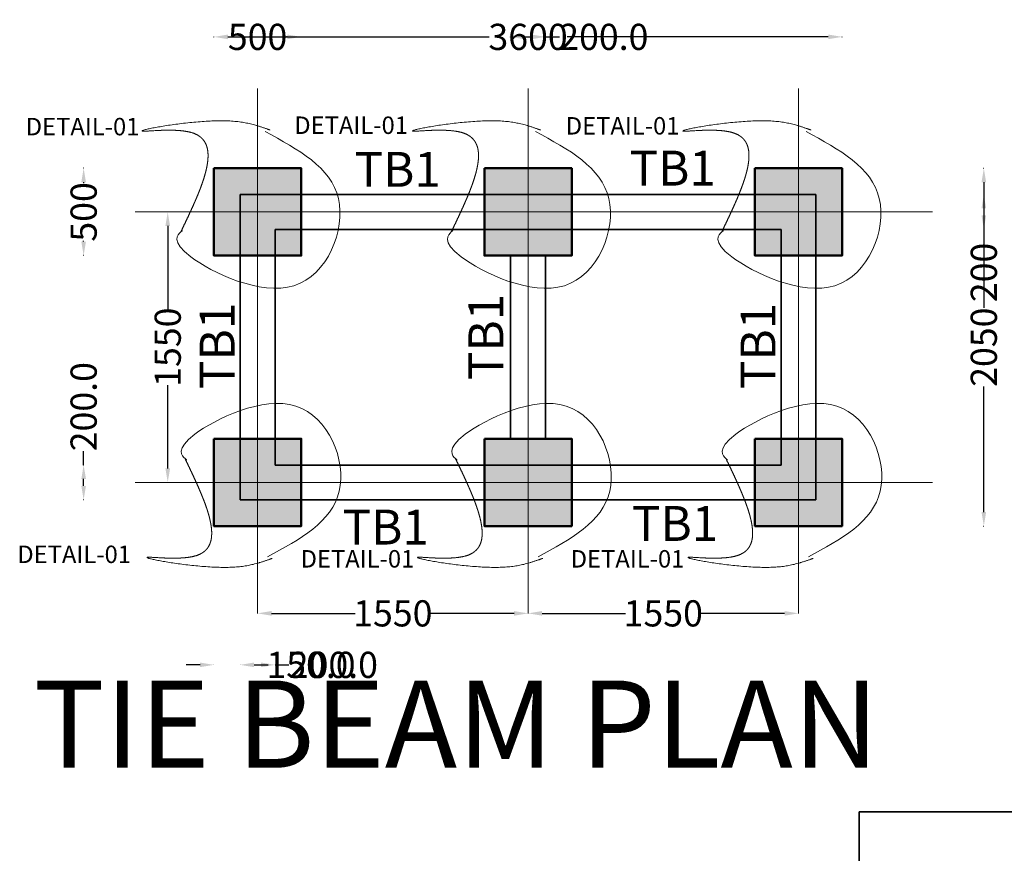
# Model space of a CAD drawing. Units: millimetres. Extents: x -19888 to 14444, y 67066 to 90098.
# Tile 5 of 7: x -13450 to -7807, y 82214 to 86990. Entities that reach past the tile are written whole.
import ezdxf

# ---------------------------------------------------------------- set-up
doc = ezdxf.new("R2010")
doc.units = ezdxf.units.MM
doc.header["$LTSCALE"] = 50
doc.header["$MEASUREMENT"] = 0
doc.linetypes.add('CENTER', pattern=[50.8, 31.75, -6.35, 6.35, -6.35])
for name, color, linetype, lineweight in [('S-ANNO-DIMS', 2, 'Continuous', 18), ('S-ANNO-SYMB', 3, 'Continuous', 18), ('S-ANNO-TEXT', 7, 'Continuous', 25), ('S-ANNO-TTLB', 7, 'Continuous', 35), ('S-BEAM', 3, 'Continuous', 35), ('S-COLS', 4, 'Continuous', 50), ('S-GRID', 8, 'CENTER', 18), ('S-PATT', 8, 'Continuous', 13)]:
    doc.layers.add(name, color=color, linetype=linetype, lineweight=lineweight)
doc.styles.get("Standard").update_dxf_attribs({"font": 'arial.ttf'})
doc.dimstyles.get("Standard").update_dxf_attribs({"dimtxt": 150, "dimasz": 80, "dimexe": 0.18, "dimexo": 0.0625, "dimgap": 0.09, "dimtad": 0, "dimdec": 0, "dimzin": 0, "dimdsep": 46, "dimtxsty": 'Standard', "dimcen": 0.09, "dimadec": 0, "dimazin": 0, "dimtfac": 1, "dimtdec": 0, "dimtofl": 0, "dimtmove": 0, "dimatfit": 3, "dimfxl": 1, "dimfxlon": 1, "dimtolj": 1, "dimtzin": 0, "dimarcsym": 0})

# ---------------------------------------------------------------- blocks, each defined once
blk = doc.blocks.new('*D16')
at = {"layer": 'Defpoints', "color": 0, "ltscale": 50, "transparency": 16777216}
for p in [(-12086.8, 83589.1), (-10536.8, 83589.1), (-10536.8, 83589.1)]:
    blk.add_point(p, dxfattribs=at)
at = {"layer": 'S-ANNO-DIMS', "color": 0, "lineweight": -2, "ltscale": 50, "transparency": 16777216}
for p, q in [((-12086.8, 83589.1), (-12086.8, 83589.3)), ((-12006.8, 83589.1), (-11528.5, 83589.1)), ((-10616.8, 83589.1), (-11095, 83589.1)), ((-10536.8, 83589.1), (-10536.8, 83589.3))]:
    blk.add_line(p, q, dxfattribs=at)
at = {"layer": 'S-ANNO-DIMS', "color": 0, "ltscale": 50, "transparency": 16777216}
for points in [[(-12006.8, 83602.4), (-12006.8, 83575.8), (-12086.8, 83589.1)], [(-10616.8, 83602.4), (-10616.8, 83575.8), (-10536.8, 83589.1)]]:
    blk.add_solid(points, dxfattribs=at)
at = {"layer": 'S-ANNO-DIMS', "color": 0, "ltscale": 50, "transparency": 16777216, "insert": (-11311.8, 83589.1), "char_height": 150, "attachment_point": 5}
blk.add_mtext('\\A1;1550', dxfattribs=at)
blk = doc.blocks.new('*D17')
at = {"layer": 'Defpoints', "color": 0, "ltscale": 50, "transparency": 16777216}
for p in [(-10536.8, 83589.3), (-8986.8, 83589.1), (-8986.8, 83589.1)]:
    blk.add_point(p, dxfattribs=at)
at = {"layer": 'S-ANNO-DIMS', "color": 0, "lineweight": -2, "ltscale": 50, "transparency": 16777216}
for p, q in [((-10536.8, 83589.2), (-10536.8, 83588.9)), ((-10456.8, 83589.1), (-9978.5, 83589.1)), ((-9066.8, 83589.1), (-9545, 83589.1)), ((-8986.8, 83589.1), (-8986.8, 83589.3))]:
    blk.add_line(p, q, dxfattribs=at)
at = {"layer": 'S-ANNO-DIMS', "color": 0, "ltscale": 50, "transparency": 16777216}
for points in [[(-10456.8, 83602.4), (-10456.8, 83575.8), (-10536.8, 83589.1)], [(-9066.8, 83602.4), (-9066.8, 83575.8), (-8986.8, 83589.1)]]:
    blk.add_solid(points, dxfattribs=at)
at = {"layer": 'S-ANNO-DIMS', "color": 0, "ltscale": 50, "transparency": 16777216, "insert": (-9761.8, 83589.1), "char_height": 150, "attachment_point": 5}
blk.add_mtext('\\A1;1550', dxfattribs=at)
blk = doc.blocks.new('*D18')
at = {"layer": 'Defpoints', "color": 0, "ltscale": 50, "transparency": 16777216}
for p in [(-12601.8, 85889.1), (-12601.8, 85889.1), (-12601.8, 84339.1)]:
    blk.add_point(p, dxfattribs=at)
at = {"layer": 'S-ANNO-DIMS', "color": 0, "lineweight": -2, "ltscale": 50, "transparency": 16777216}
for p, q in [((-12601.8, 85889.1), (-12601.9, 85889.1)), ((-12601.8, 85809.1), (-12601.8, 85330.9)), ((-12601.8, 84419.1), (-12601.8, 84897.4)), ((-12601.8, 84339.1), (-12601.9, 84339.1))]:
    blk.add_line(p, q, dxfattribs=at)
at = {"layer": 'S-ANNO-DIMS', "color": 0, "ltscale": 50, "transparency": 16777216}
for points in [[(-12615.1, 85809.1), (-12588.4, 85809.1), (-12601.8, 85889.1)], [(-12615.1, 84419.1), (-12588.4, 84419.1), (-12601.8, 84339.1)]]:
    blk.add_solid(points, dxfattribs=at)
at = {"layer": 'S-ANNO-DIMS', "color": 0, "ltscale": 50, "transparency": 16777216, "insert": (-12601.8, 85114.1), "char_height": 150, "attachment_point": 5, "rotation": 90}
blk.add_mtext('\\A1;1550', dxfattribs=at)
blk = doc.blocks.new('*D28')
at = {"layer": 'Defpoints', "color": 0, "ltscale": 50, "transparency": 16777216}
for p in [(-11836.8, 86892), (-12336.8, 86139.1), (-11836.8, 86139.1)]:
    blk.add_point(p, dxfattribs=at)
at = {"layer": 'S-ANNO-DIMS', "color": 0, "lineweight": -2, "ltscale": 50, "transparency": 16777216}
for p, q in [((-12336.8, 86891), (-12336.8, 86892.2)), ((-12256.8, 86892), (-12252.3, 86892)), ((-11916.8, 86892), (-11921.2, 86892)), ((-11836.8, 86891), (-11836.8, 86892.2))]:
    blk.add_line(p, q, dxfattribs=at)
at = {"layer": 'S-ANNO-DIMS', "color": 0, "ltscale": 50, "transparency": 16777216}
for points in [[(-12256.8, 86905.3), (-12256.8, 86878.6), (-12336.8, 86892)], [(-11916.8, 86905.3), (-11916.8, 86878.6), (-11836.8, 86892)]]:
    blk.add_solid(points, dxfattribs=at)
at = {"layer": 'S-ANNO-DIMS', "color": 0, "ltscale": 50, "transparency": 16777216, "insert": (-12086.8, 86892), "char_height": 150, "attachment_point": 5}
blk.add_mtext('\\A1;500', dxfattribs=at)
blk = doc.blocks.new('*D29')
at = {"layer": 'Defpoints', "color": 0, "ltscale": 50, "transparency": 16777216}
for p in [(-12336.8, 86139.1), (-13083.7, 85639.1), (-12336.8, 85639.1)]:
    blk.add_point(p, dxfattribs=at)
at = {"layer": 'S-ANNO-DIMS', "color": 0, "lineweight": -2, "ltscale": 50, "transparency": 16777216}
for p, q in [((-13082.7, 86139.1), (-13083.8, 86139.1)), ((-13083.7, 86059.1), (-13083.7, 86054.6)), ((-13083.7, 85719.1), (-13083.7, 85723.6)), ((-13082.7, 85639.1), (-13083.8, 85639.1))]:
    blk.add_line(p, q, dxfattribs=at)
at = {"layer": 'S-ANNO-DIMS', "color": 0, "ltscale": 50, "transparency": 16777216}
for points in [[(-13097, 86059.1), (-13070.3, 86059.1), (-13083.7, 86139.1)], [(-13097, 85719.1), (-13070.3, 85719.1), (-13083.7, 85639.1)]]:
    blk.add_solid(points, dxfattribs=at)
at = {"layer": 'S-ANNO-DIMS', "color": 0, "ltscale": 50, "transparency": 16777216, "insert": (-13083.7, 85889.1), "char_height": 150, "attachment_point": 5, "rotation": 90}
blk.add_mtext('\\A1;500', dxfattribs=at)
blk = doc.blocks.new('*D30')
at = {"layer": 'Defpoints', "color": 0, "ltscale": 50, "transparency": 16777216}
for p in [(-8736.8, 86892), (-12336.8, 86139.1), (-8736.8, 86139.1)]:
    blk.add_point(p, dxfattribs=at)
at = {"layer": 'S-ANNO-DIMS', "color": 0, "lineweight": -2, "ltscale": 50, "transparency": 16777216}
for p, q in [((-12336.8, 86891), (-12336.8, 86892.2)), ((-12256.8, 86892), (-10760.5, 86892)), ((-8816.8, 86892), (-10313, 86892)), ((-8736.8, 86891), (-8736.8, 86892.2))]:
    blk.add_line(p, q, dxfattribs=at)
at = {"layer": 'S-ANNO-DIMS', "color": 0, "ltscale": 50, "transparency": 16777216}
for points in [[(-12256.8, 86905.3), (-12256.8, 86878.6), (-12336.8, 86892)], [(-8816.8, 86905.3), (-8816.8, 86878.6), (-8736.8, 86892)]]:
    blk.add_solid(points, dxfattribs=at)
at = {"layer": 'S-ANNO-DIMS', "color": 0, "ltscale": 50, "transparency": 16777216, "insert": (-10536.8, 86892), "char_height": 150, "attachment_point": 5}
blk.add_mtext('\\A1;3600', dxfattribs=at)
blk = doc.blocks.new('*D31')
at = {"layer": 'Defpoints', "color": 0, "ltscale": 50, "transparency": 16777216}
for p in [(-8736.8, 86139.1), (-8736.8, 84089.1), (-7924.9, 84089.1)]:
    blk.add_point(p, dxfattribs=at)
at = {"layer": 'S-ANNO-DIMS', "color": 0, "lineweight": -2, "ltscale": 50, "transparency": 16777216}
for p, q in [((-7925.9, 86139.1), (-7924.7, 86139.1)), ((-7924.9, 86059.1), (-7924.9, 85339.2)), ((-7924.9, 84169.1), (-7924.9, 84889)), ((-7925.9, 84089.1), (-7924.7, 84089.1))]:
    blk.add_line(p, q, dxfattribs=at)
at = {"layer": 'S-ANNO-DIMS', "color": 0, "ltscale": 50, "transparency": 16777216}
for points in [[(-7938.2, 86059.1), (-7911.5, 86059.1), (-7924.9, 86139.1)], [(-7938.2, 84169.1), (-7911.5, 84169.1), (-7924.9, 84089.1)]]:
    blk.add_solid(points, dxfattribs=at)
at = {"layer": 'S-ANNO-DIMS', "color": 0, "ltscale": 50, "transparency": 16777216, "insert": (-7924.9, 85114.1), "char_height": 150, "attachment_point": 5, "rotation": 90}
blk.add_mtext('\\A1;2050', dxfattribs=at)
blk = doc.blocks.new('*D32')
at = {"layer": 'Defpoints', "color": 0, "ltscale": 50, "transparency": 16777216}
for p in [(-12186.8, 85989.1), (-11986.8, 85789.1), (-7924.9, 85789.1)]:
    blk.add_point(p, dxfattribs=at)
at = {"layer": 'S-ANNO-DIMS', "color": 0, "lineweight": -2, "ltscale": 50, "transparency": 16777216}
for p, q in [((-7925.9, 85989.1), (-7924.7, 85989.1)), ((-7924.9, 85909.1), (-7924.9, 85869.1)), ((-7925.9, 85789.1), (-7924.7, 85789.1)), ((-7924.9, 85789.1), (-7924.9, 85709.1))]:
    blk.add_line(p, q, dxfattribs=at)
at = {"layer": 'S-ANNO-DIMS', "color": 0, "ltscale": 50, "transparency": 16777216}
for points in [[(-7938.2, 85909.1), (-7911.5, 85909.1), (-7924.9, 85989.1)], [(-7938.2, 85869.1), (-7911.5, 85869.1), (-7924.9, 85789.1)]]:
    blk.add_solid(points, dxfattribs=at)
at = {"layer": 'S-ANNO-DIMS', "color": 0, "ltscale": 50, "transparency": 16777216, "insert": (-7924.9, 85542.3), "char_height": 150, "attachment_point": 5, "rotation": 90}
blk.add_mtext('\\A1;200', dxfattribs=at)
blk = doc.blocks.new('*D76')
at = {"layer": 'Defpoints', "color": 0, "ltscale": 50, "transparency": 16777216}
for p in [(-10436.8, 86892), (-10636.8, 85639.1), (-10436.8, 85639.1)]:
    blk.add_point(p, dxfattribs=at)
at = {"layer": 'S-ANNO-DIMS', "color": 0, "lineweight": -2, "ltscale": 50, "transparency": 16777216}
for p, q in [((-10636.8, 86891), (-10636.8, 86892.2)), ((-10556.8, 86892), (-10516.8, 86892)), ((-10436.8, 86891), (-10436.8, 86892.2)), ((-10436.8, 86892), (-10356.8, 86892))]:
    blk.add_line(p, q, dxfattribs=at)
at = {"layer": 'S-ANNO-DIMS', "color": 0, "ltscale": 50, "transparency": 16777216}
for points in [[(-10556.8, 86905.3), (-10556.8, 86878.6), (-10636.8, 86892)], [(-10516.8, 86905.3), (-10516.8, 86878.6), (-10436.8, 86892)]]:
    blk.add_solid(points, dxfattribs=at)
at = {"layer": 'S-ANNO-DIMS', "color": 0, "ltscale": 50, "transparency": 16777216, "insert": (-10102.6, 86892), "char_height": 150, "attachment_point": 5}
blk.add_mtext('\\A1;200.0', dxfattribs=at)
blk = doc.blocks.new('*D77')
at = {"layer": 'Defpoints', "color": 0, "ltscale": 50, "transparency": 16777216}
for p in [(-13083.7, 84439.1), (-11986.8, 84439.1), (-12186.8, 84239.1)]:
    blk.add_point(p, dxfattribs=at)
at = {"layer": 'S-ANNO-DIMS', "color": 0, "lineweight": -2, "ltscale": 50, "transparency": 16777216}
for p, q in [((-13083.7, 84439.1), (-13083.7, 84519.1)), ((-13082.7, 84439.1), (-13083.8, 84439.1)), ((-13083.7, 84319.1), (-13083.7, 84359.1)), ((-13082.7, 84239.1), (-13083.8, 84239.1))]:
    blk.add_line(p, q, dxfattribs=at)
at = {"layer": 'S-ANNO-DIMS', "color": 0, "ltscale": 50, "transparency": 16777216}
for points in [[(-13097, 84359.1), (-13070.3, 84359.1), (-13083.7, 84439.1)], [(-13097, 84319.1), (-13070.3, 84319.1), (-13083.7, 84239.1)]]:
    blk.add_solid(points, dxfattribs=at)
at = {"layer": 'S-ANNO-DIMS', "color": 0, "ltscale": 50, "transparency": 16777216, "insert": (-13083.7, 84773.3), "char_height": 150, "attachment_point": 5, "rotation": 90}
blk.add_mtext('\\A1;200.0', dxfattribs=at)
blk = doc.blocks.new('*D78')
at = {"layer": 'Defpoints', "color": 0, "ltscale": 50, "transparency": 16777216}
for p in [(-11986.8, 84439.1), (-12186.8, 84239.1), (-11986.8, 83294.1)]:
    blk.add_point(p, dxfattribs=at)
at = {"layer": 'S-ANNO-DIMS', "color": 0, "lineweight": -2, "ltscale": 50, "transparency": 16777216}
for p, q in [((-12186.8, 83295.1), (-12186.8, 83293.9)), ((-12106.8, 83294.1), (-12066.8, 83294.1)), ((-11986.8, 83295.1), (-11986.8, 83293.9)), ((-11986.8, 83294.1), (-11906.8, 83294.1))]:
    blk.add_line(p, q, dxfattribs=at)
at = {"layer": 'S-ANNO-DIMS', "color": 0, "ltscale": 50, "transparency": 16777216}
for points in [[(-12106.8, 83307.4), (-12106.8, 83280.8), (-12186.8, 83294.1)], [(-12066.8, 83307.4), (-12066.8, 83280.8), (-11986.8, 83294.1)]]:
    blk.add_solid(points, dxfattribs=at)
at = {"layer": 'S-ANNO-DIMS', "color": 0, "ltscale": 50, "transparency": 16777216, "insert": (-11652.6, 83294.1), "char_height": 150, "attachment_point": 5}
blk.add_mtext('\\A1;200.0', dxfattribs=at)
blk = doc.blocks.new('*D79')
at = {"layer": 'Defpoints', "color": 0, "ltscale": 50, "transparency": 16777216}
for p in [(-12186.8, 84239.1), (-12336.8, 84089.1), (-12186.8, 83294.1)]:
    blk.add_point(p, dxfattribs=at)
at = {"layer": 'S-ANNO-DIMS', "color": 0, "lineweight": -2, "ltscale": 50, "transparency": 16777216}
for p, q in [((-12416.8, 83294.1), (-12496.8, 83294.1)), ((-12336.8, 83295.1), (-12336.8, 83293.9)), ((-12186.8, 83295.1), (-12186.8, 83293.9)), ((-12106.8, 83294.1), (-12026.8, 83294.1))]:
    blk.add_line(p, q, dxfattribs=at)
at = {"layer": 'S-ANNO-DIMS', "color": 0, "ltscale": 50, "transparency": 16777216}
for points in [[(-12416.8, 83307.4), (-12416.8, 83280.8), (-12336.8, 83294.1)], [(-12106.8, 83307.4), (-12106.8, 83280.8), (-12186.8, 83294.1)]]:
    blk.add_solid(points, dxfattribs=at)
at = {"layer": 'S-ANNO-DIMS', "color": 0, "ltscale": 50, "transparency": 16777216, "insert": (-11780.9, 83294.1), "char_height": 150, "attachment_point": 5}
blk.add_mtext('\\A1;150.0', dxfattribs=at)

msp = doc.modelspace()

# ---------------------------------------------------------------- hatches: boundary and pattern name
at = {"layer": 'S-PATT', "ltscale": 50}
h = msp.add_hatch(dxfattribs=at)
h.set_pattern_fill('AR-SAND', color=256, scale=30)
h.set_pattern_definition([(37.5, (-1279.46, 831.89), (-1.8898, 57.804713), [0, -45.6, 0, -51, 0, -48.75]), (7.5, (-1279.46, 831.89), (53.0933, 84.66438), [0, -24.6, 0, -41.1, 0, -15.75]), (327.5, (-1316.36, 831.89), (93.424256, 0.169772), [0, -15, 0, -54, 0, -70.5]), (317.5, (-1316.36, 831.89), (90.1838, 26.33027), [0, -7.5, 0, -35.4, 0, -40.5])])
h.paths.add_polyline_path([(-11836.756, 86139.101), (-12086.756, 86139.101), (-12086.756, 85989.101), (-11836.756, 85989.101)])
h.paths.add_polyline_path([(-12086.756, 86139.101), (-12336.756, 86139.101), (-12336.756, 85889.101), (-12186.756, 85889.101), (-12186.756, 85989.101), (-12086.756, 85989.101)])
h.paths.add_polyline_path([(-12186.756, 85889.101), (-12336.756, 85889.101), (-12336.756, 85639.101), (-12186.756, 85639.101)])
h.paths.add_polyline_path([(-12086.756, 85989.101), (-12186.756, 85989.101), (-12186.756, 85889.101), (-12086.756, 85889.101)], flags=17)
h.paths.add_polyline_path([(-12086.756, 85889.101), (-12186.756, 85889.101), (-12186.756, 85639.101), (-12086.756, 85639.101)])
h.paths.add_polyline_path([(-11836.756, 85889.101), (-12086.756, 85889.101), (-12086.756, 85639.101), (-11986.756, 85639.101), (-11986.756, 85789.101), (-11836.756, 85789.101)])
h.paths.add_polyline_path([(-11836.756, 85789.101), (-11986.756, 85789.101), (-11986.756, 85639.101), (-11836.756, 85639.101)], flags=17)
h.paths.add_polyline_path([(-11836.756, 85989.101), (-12086.756, 85989.101), (-12086.756, 85889.101), (-11836.756, 85889.101)])
h.paths.add_polyline_path([(-10536.756, 86139.101), (-10786.756, 86139.101), (-10786.756, 85989.101), (-10536.756, 85989.101)])
h.paths.add_polyline_path([(-10286.756, 86139.101), (-10536.756, 86139.101), (-10536.756, 85989.101), (-10286.756, 85989.101)])
h.paths.add_polyline_path([(-10286.756, 85989.101), (-10536.756, 85989.101), (-10536.756, 85889.101), (-10286.756, 85889.101)])
h.paths.add_polyline_path([(-10286.756, 85889.101), (-10536.756, 85889.101), (-10786.756, 85889.101), (-10786.756, 85639.101), (-10286.756, 85639.101)])
h.paths.add_polyline_path([(-10536.756, 85989.101), (-10786.756, 85989.101), (-10786.756, 85889.101), (-10536.756, 85889.101)])
h.paths.add_polyline_path([(-8736.756, 86139.101), (-8986.756, 86139.101), (-8986.756, 85989.101), (-8886.756, 85989.101), (-8886.756, 85889.101), (-8736.756, 85889.101)])
h.paths.add_polyline_path([(-8736.756, 85889.101), (-8886.756, 85889.101), (-8886.756, 85639.101), (-8736.756, 85639.101)])
h.paths.add_polyline_path([(-8886.756, 85889.101), (-8986.756, 85889.101), (-8986.756, 85639.101), (-8886.756, 85639.101)])
h.paths.add_polyline_path([(-8886.756, 85989.101), (-8986.756, 85989.101), (-8986.756, 85889.101), (-8886.756, 85889.101)], flags=17)
h.paths.add_polyline_path([(-8986.756, 85989.101), (-9236.756, 85989.101), (-9236.756, 85889.101), (-8986.756, 85889.101)])
h.paths.add_polyline_path([(-8986.756, 85889.101), (-9236.756, 85889.101), (-9236.756, 85789.101), (-9086.756, 85789.101), (-9086.756, 85639.101), (-8986.756, 85639.101)])
h.paths.add_polyline_path([(-9086.756, 85789.101), (-9236.756, 85789.101), (-9236.756, 85639.101), (-9086.756, 85639.101)], flags=17)
h.paths.add_polyline_path([(-8986.756, 86139.101), (-9236.756, 86139.101), (-9236.756, 85989.101), (-8986.756, 85989.101)])
h.paths.add_polyline_path([(-8736.756, 84589.101), (-8886.756, 84589.101), (-8886.756, 84339.101), (-8736.756, 84339.101)])
h.paths.add_polyline_path([(-8736.756, 84339.101), (-8886.756, 84339.101), (-8886.756, 84239.101), (-8986.756, 84239.101), (-8986.756, 84089.101), (-8736.756, 84089.101)])
h.paths.add_polyline_path([(-8986.756, 84239.101), (-9236.756, 84239.101), (-9236.756, 84089.101), (-8986.756, 84089.101)])
h.paths.add_polyline_path([(-8986.756, 84339.101), (-9236.756, 84339.101), (-9236.756, 84239.101), (-8986.756, 84239.101)])
h.paths.add_polyline_path([(-8886.756, 84339.101), (-8986.756, 84339.101), (-8986.756, 84239.101), (-8886.756, 84239.101)])
h.paths.add_polyline_path([(-8886.756, 84589.101), (-8986.756, 84589.101), (-8986.756, 84339.101), (-8886.756, 84339.101)])
h.paths.add_polyline_path([(-8986.756, 84589.101), (-9086.756, 84589.101), (-9086.756, 84439.101), (-9236.756, 84439.101), (-9236.756, 84339.101), (-8986.756, 84339.101)])
h.paths.add_polyline_path([(-9086.756, 84589.101), (-9236.756, 84589.101), (-9236.756, 84439.101), (-9086.756, 84439.101)], flags=17)
h.paths.add_polyline_path([(-10286.756, 84589.101), (-10536.756, 84589.101), (-10536.756, 84439.101), (-10286.756, 84439.101)])
h.paths.add_polyline_path([(-10536.756, 84589.101), (-10786.756, 84589.101), (-10786.756, 84439.101), (-10536.756, 84439.101)])
h.paths.add_polyline_path([(-10536.756, 84439.101), (-10786.756, 84439.101), (-10786.756, 84339.101), (-10536.756, 84339.101)])
h.paths.add_polyline_path([(-10286.756, 84439.101), (-10536.756, 84439.101), (-10536.756, 84339.101), (-10286.756, 84339.101)])
h.paths.add_polyline_path([(-10286.756, 84339.101), (-10536.756, 84339.101), (-10536.756, 84239.101), (-10286.756, 84239.101)])
h.paths.add_polyline_path([(-10286.756, 84239.101), (-10536.756, 84239.101), (-10536.756, 84089.101), (-10286.756, 84089.101)])
h.paths.add_polyline_path([(-10536.756, 84239.101), (-10786.756, 84239.101), (-10786.756, 84089.101), (-10536.756, 84089.101)])
h.paths.add_polyline_path([(-10536.756, 84339.101), (-10786.756, 84339.101), (-10786.756, 84239.101), (-10536.756, 84239.101)])
h.paths.add_polyline_path([(-11836.756, 84589.101), (-11986.756, 84589.101), (-11986.756, 84439.101), (-11836.756, 84439.101)], flags=17)
h.paths.add_polyline_path([(-11836.756, 84439.101), (-11986.756, 84439.101), (-11986.756, 84589.101), (-12086.756, 84589.101), (-12086.756, 84339.101), (-11836.756, 84339.101)])
h.paths.add_polyline_path([(-12086.756, 84589.101), (-12186.756, 84589.101), (-12186.756, 84339.101), (-12086.756, 84339.101)])
h.paths.add_polyline_path([(-12186.756, 84589.101), (-12336.756, 84589.101), (-12336.756, 84339.101), (-12186.756, 84339.101)])
h.paths.add_polyline_path([(-12086.756, 84239.101), (-12186.756, 84239.101), (-12186.756, 84339.101), (-12336.756, 84339.101), (-12336.756, 84089.101), (-12086.756, 84089.101)])
h.paths.add_polyline_path([(-12086.756, 84339.101), (-12186.756, 84339.101), (-12186.756, 84239.101), (-12086.756, 84239.101)], flags=17)
h.paths.add_polyline_path([(-11836.756, 84339.101), (-12086.756, 84339.101), (-12086.756, 84239.101), (-11836.756, 84239.101)])
h.paths.add_polyline_path([(-11836.756, 84239.101), (-12086.756, 84239.101), (-12086.756, 84089.101), (-11836.756, 84089.101)])

# ---------------------------------------------------------------- linework, layer by layer
at = {"layer": 'S-ANNO-SYMB', "ltscale": 50}
for points in [[(-12016.027, 86358.35), (-12077.072, 86380.249), (-12284.841, 86454.784), (-13003.704, 86314.412), (-12221.183, 86410.387), (-12404.949, 86028.076), (-12528.19, 85771.685), (-12536.302, 85714.276), (-12512.9, 85661.229), (-12465.03, 85628.517), (-12417.161, 85595.805), (-12359.237, 85593.277), (-12308.699, 85621.694), (-12269.374, 85527.391), (-12177.953, 85481.768), (-12078.955, 85507.041), (-12052.393, 85472.909), (-12014.594, 85451.892), (-11971.584, 85447.339), (-11928.575, 85442.786), (-11887.213, 85455.424), (-11854.093, 85483.237), (-11785.59, 85469.564), (-11719.137, 85491.097), (-11671.671, 85542.347), (-11624.205, 85593.598), (-11607.824, 85661.504), (-11626.701, 85728.759), (-11587.457, 85760.162), (-11566.838, 85806), (-11569.374, 85856.198), (-11571.91, 85906.396), (-11597.044, 85949.922), (-11639.254, 85977.21), (-11638.25, 86024.51), (-11656.94, 86067.974), (-11691.962, 86099.783), (-11726.983, 86131.592), (-11772.039, 86146.026), (-11819.025, 86140.49), (-11802.373, 86204.037), (-11820.704, 86267.121), (-11868.82, 86311.847), (-11916.936, 86356.573), (-11981.188, 86370.255), (-12043.351, 86349.012)], [(-10466.027, 86358.35), (-10527.072, 86380.249), (-10734.841, 86454.784), (-11453.704, 86314.412), (-10671.183, 86410.387), (-10854.949, 86028.076), (-10978.19, 85771.685), (-10986.302, 85714.276), (-10962.9, 85661.229), (-10915.03, 85628.517), (-10867.161, 85595.805), (-10809.237, 85593.277), (-10758.699, 85621.694), (-10719.374, 85527.391), (-10627.953, 85481.768), (-10528.955, 85507.041), (-10502.393, 85472.909), (-10464.594, 85451.892), (-10421.584, 85447.339), (-10378.575, 85442.786), (-10337.213, 85455.424), (-10304.093, 85483.237), (-10235.59, 85469.564), (-10169.137, 85491.097), (-10121.671, 85542.347), (-10074.205, 85593.598), (-10057.824, 85661.504), (-10076.701, 85728.759), (-10037.457, 85760.162), (-10016.838, 85806), (-10019.374, 85856.198), (-10021.91, 85906.396), (-10047.044, 85949.922), (-10089.254, 85977.21), (-10088.25, 86024.51), (-10106.94, 86067.974), (-10141.962, 86099.783), (-10176.983, 86131.592), (-10222.039, 86146.026), (-10269.025, 86140.49), (-10252.373, 86204.037), (-10270.704, 86267.121), (-10318.82, 86311.847), (-10366.936, 86356.573), (-10431.188, 86370.255), (-10493.351, 86349.012)], [(-8916.027, 86358.35), (-8977.072, 86380.249), (-9184.841, 86454.784), (-9903.704, 86314.412), (-9121.183, 86410.387), (-9304.949, 86028.076), (-9428.19, 85771.685), (-9436.302, 85714.276), (-9412.9, 85661.229), (-9365.03, 85628.517), (-9317.161, 85595.805), (-9259.237, 85593.277), (-9208.699, 85621.694), (-9169.374, 85527.391), (-9077.953, 85481.768), (-8978.955, 85507.041), (-8952.393, 85472.909), (-8914.594, 85451.892), (-8871.584, 85447.339), (-8828.575, 85442.786), (-8787.213, 85455.424), (-8754.093, 85483.237), (-8685.59, 85469.564), (-8619.137, 85491.097), (-8571.671, 85542.347), (-8524.205, 85593.598), (-8507.824, 85661.504), (-8526.701, 85728.759), (-8487.457, 85760.162), (-8466.838, 85806), (-8469.374, 85856.198), (-8471.91, 85906.396), (-8497.044, 85949.922), (-8539.254, 85977.21), (-8538.25, 86024.51), (-8556.94, 86067.974), (-8591.962, 86099.783), (-8626.983, 86131.592), (-8672.039, 86146.026), (-8719.025, 86140.49), (-8702.373, 86204.037), (-8720.704, 86267.121), (-8768.82, 86311.847), (-8816.936, 86356.573), (-8881.188, 86370.255), (-8943.351, 86349.012)], [(-12002.702, 83904.311), (-12062.445, 83882.879), (-12265.782, 83809.934), (-12969.308, 83947.311), (-12203.481, 83853.384), (-12383.327, 84227.538), (-12503.939, 84478.46), (-12511.878, 84534.644), (-12488.975, 84586.559), (-12442.126, 84618.573), (-12395.278, 84650.587), (-12338.59, 84653.061), (-12289.13, 84625.251), (-12250.645, 84717.541), (-12161.174, 84762.191), (-12064.288, 84737.457), (-12038.292, 84770.861), (-12001.3, 84791.43), (-11959.208, 84795.886), (-11917.116, 84800.342), (-11876.636, 84787.974), (-11844.223, 84760.753), (-11777.181, 84774.134), (-11712.147, 84753.061), (-11665.693, 84702.904), (-11619.24, 84652.747), (-11603.208, 84586.29), (-11621.683, 84520.47), (-11583.276, 84489.736), (-11563.096, 84444.877), (-11565.578, 84395.75), (-11568.06, 84346.623), (-11592.659, 84304.025), (-11633.967, 84277.319), (-11632.985, 84231.028), (-11651.276, 84188.492), (-11685.551, 84157.361), (-11719.825, 84126.231), (-11763.92, 84112.104), (-11809.903, 84117.522), (-11793.606, 84055.331), (-11811.546, 83993.594), (-11858.636, 83949.822), (-11905.725, 83906.05), (-11968.606, 83892.66), (-12029.444, 83913.449)], [(-10452.702, 83904.311), (-10512.445, 83882.879), (-10715.782, 83809.934), (-11419.308, 83947.311), (-10653.481, 83853.384), (-10833.327, 84227.538), (-10953.939, 84478.46), (-10961.878, 84534.644), (-10938.975, 84586.559), (-10892.126, 84618.573), (-10845.278, 84650.587), (-10788.59, 84653.061), (-10739.13, 84625.251), (-10700.645, 84717.541), (-10611.174, 84762.191), (-10514.288, 84737.457), (-10488.292, 84770.861), (-10451.3, 84791.43), (-10409.208, 84795.886), (-10367.116, 84800.342), (-10326.636, 84787.974), (-10294.223, 84760.753), (-10227.181, 84774.134), (-10162.147, 84753.061), (-10115.693, 84702.904), (-10069.24, 84652.747), (-10053.208, 84586.29), (-10071.683, 84520.47), (-10033.276, 84489.736), (-10013.096, 84444.877), (-10015.578, 84395.75), (-10018.06, 84346.623), (-10042.659, 84304.025), (-10083.967, 84277.319), (-10082.985, 84231.028), (-10101.276, 84188.492), (-10135.551, 84157.361), (-10169.825, 84126.231), (-10213.92, 84112.104), (-10259.903, 84117.522), (-10243.606, 84055.331), (-10261.546, 83993.594), (-10308.636, 83949.822), (-10355.725, 83906.05), (-10418.606, 83892.66), (-10479.444, 83913.449)], [(-8902.702, 83904.311), (-8962.445, 83882.879), (-9165.782, 83809.934), (-9869.308, 83947.311), (-9103.481, 83853.384), (-9283.327, 84227.538), (-9403.939, 84478.46), (-9411.878, 84534.644), (-9388.975, 84586.559), (-9342.126, 84618.573), (-9295.278, 84650.587), (-9238.59, 84653.061), (-9189.13, 84625.251), (-9150.645, 84717.541), (-9061.174, 84762.191), (-8964.288, 84737.457), (-8938.292, 84770.861), (-8901.3, 84791.43), (-8859.208, 84795.886), (-8817.116, 84800.342), (-8776.636, 84787.974), (-8744.223, 84760.753), (-8677.181, 84774.134), (-8612.147, 84753.061), (-8565.693, 84702.904), (-8519.24, 84652.747), (-8503.208, 84586.29), (-8521.683, 84520.47), (-8483.276, 84489.736), (-8463.096, 84444.877), (-8465.578, 84395.75), (-8468.06, 84346.623), (-8492.659, 84304.025), (-8533.967, 84277.319), (-8532.985, 84231.028), (-8551.276, 84188.492), (-8585.551, 84157.361), (-8619.825, 84126.231), (-8663.92, 84112.104), (-8709.903, 84117.522), (-8693.606, 84055.331), (-8711.546, 83993.594), (-8758.636, 83949.822), (-8805.725, 83906.05), (-8868.606, 83892.66), (-8929.444, 83913.449)]]:
    msp.add_rational_spline(points, [1, 1, 1, 1, 1, 1, 1, 0.899635465557, 0.899635465557, 1, 0.899635465557, 0.899635465557, 1, 0.837674523405, 0.837674523405, 1, 0.946853392125, 0.946853392125, 1, 0.946853392125, 0.946853392125, 1, 0.915045194392, 0.915045194392, 1, 0.915045194392, 0.915045194392, 1, 0.926742131358, 0.926742131358, 1, 0.926742131358, 0.926742131358, 1, 0.940052407466, 0.940052407466, 1, 0.940052407466, 0.940052407466, 1, 0.905450537791, 0.905450537791, 1, 0.905450537791, 0.905450537791, 1], degree=3, knots=[0, 0, 0, 0, 316.97779253, 1078.83968779, 1492.74004437, 2335.50803491, 2335.50803491, 2335.50803491, 2336.61973124, 2336.61973124, 2336.61973124, 2337.73142758, 2337.73142758, 2337.73142758, 2339.15709482, 2339.15709482, 2339.15709482, 2339.96109598, 2339.96109598, 2339.96109598, 2340.76509714, 2340.76509714, 2340.76509714, 2341.78582089, 2341.78582089, 2341.78582089, 2342.80654464, 2342.80654464, 2342.80654464, 2343.75295031, 2343.75295031, 2343.75295031, 2344.69935599, 2344.69935599, 2344.69935599, 2345.55400123, 2345.55400123, 2345.55400123, 2346.40864648, 2346.40864648, 2346.40864648, 2347.48682797, 2347.48682797, 2347.48682797, 2348.56500946, 2348.56500946, 2348.56500946, 2348.56500946], dxfattribs=at)
at = {"layer": 'S-ANNO-TTLB', "ltscale": 50}
msp.add_lwpolyline([(-8639.597, 82452.304), (5654.103, 82452.304), (5654.103, 77078.62), (-8639.597, 77078.62)], close=True, dxfattribs=at)
at = {"layer": 'S-BEAM', "ltscale": 50}
for p, q in [((-12186.756, 85989.101), (-8886.756, 85989.101)), ((-12186.756, 85989.101), (-12186.756, 84239.101)), ((-8886.756, 85989.101), (-8886.756, 84239.101)), ((-11986.756, 85789.101), (-9086.756, 85789.101)), ((-11986.756, 85789.101), (-11986.756, 84439.101)), ((-9086.756, 85789.101), (-9086.756, 84439.101)), ((-10636.756, 85639.101), (-10636.756, 84589.101)), ((-10436.756, 85639.101), (-10436.756, 84589.101)), ((-11986.756, 84439.101), (-9086.756, 84439.101)), ((-12186.756, 84239.101), (-8886.756, 84239.101))]:
    msp.add_line(p, q, dxfattribs=at)
at = {"layer": 'S-COLS', "ltscale": 50}
for points in [[(-12336.756, 86139.101), (-11836.756, 86139.101), (-11836.756, 85639.101), (-12336.756, 85639.101)], [(-10786.756, 86139.101), (-10286.756, 86139.101), (-10286.756, 85639.101), (-10786.756, 85639.101)], [(-9236.756, 86139.101), (-8736.756, 86139.101), (-8736.756, 85639.101), (-9236.756, 85639.101)], [(-12336.756, 84589.101), (-11836.756, 84589.101), (-11836.756, 84089.101), (-12336.756, 84089.101)], [(-10786.756, 84589.101), (-10286.756, 84589.101), (-10286.756, 84089.101), (-10786.756, 84089.101)], [(-9236.756, 84589.101), (-8736.756, 84589.101), (-8736.756, 84089.101), (-9236.756, 84089.101)]]:
    msp.add_lwpolyline(points, close=True, dxfattribs=at)
at = {"layer": 'S-GRID', "ltscale": 50}
for p, q in [((-12086.756, 85889.101), (-12086.756, 86596.981)), ((-10536.756, 85639.101), (-10536.756, 86596.981)), ((-8986.756, 85889.101), (-8986.756, 86596.981)), ((-12086.756, 85889.101), (-12788.669, 85889.101)), ((-12086.756, 85889.101), (-12086.756, 84339.101)), ((-12086.756, 85889.101), (-8986.756, 85889.101)), ((-8986.756, 85889.101), (-8986.756, 84339.101)), ((-8986.756, 85889.101), (-8219.875, 85889.101)), ((-10536.756, 85639.101), (-10536.756, 84589.101)), ((-10536.756, 84589.101), (-10536.756, 83589.101)), ((-12086.756, 84339.101), (-12788.669, 84339.101)), ((-12086.756, 84339.101), (-8986.756, 84339.101)), ((-12086.756, 84339.101), (-12086.756, 83589.101)), ((-8986.756, 84339.101), (-8986.756, 83589.101)), ((-8986.756, 84339.101), (-8219.875, 84339.101))]:
    msp.add_line(p, q, dxfattribs=at)

# ---------------------------------------------------------------- texts
at = {"layer": 'S-ANNO-TEXT', "ltscale": 50, "attachment_point": 1}
for s, width, insert, char_height in [('DETAIL-01', 1609.35955, (-13415.712, 86427.877), 100), ('DETAIL-01', 1609.35955, (-11876.656, 86435.851), 100), ('DETAIL-01', 1609.35955, (-10320.887, 86432.42), 100), ('TB1', 1609.35955, (-11530.914, 86233.014), 200), ('TB1', 1609.35955, (-9954.859, 86239.858), 200), ('TB1', 1609.35955, (-9941.224, 84204.155), 200), ('TB1', 1609.35955, (-11599.508, 84183.623), 200), ('DETAIL-01', 1609.35955, (-13463.923, 83977.397), 100), ('DETAIL-01', 1609.35955, (-11840.351, 83951.562), 100), ('DETAIL-01', 1609.35955, (-10292.651, 83951.457), 100), ('TIE BEAM PLAN', 5845.79275, (-13370.787, 83204.308), 500)]:
    msp.add_mtext_dynamic_manual_height_columns(s, width=width, gutter_width=1, heights=[0], dxfattribs=dict(at, insert=insert, char_height=char_height))
at = {"layer": 'S-ANNO-TEXT', "ltscale": 50, "char_height": 200, "attachment_point": 1, "rotation": 90}
for insert in [(-10878.602, 84925.724), (-12418.434, 84874.684), (-9318.864, 84874.227)]:
    msp.add_mtext_dynamic_manual_height_columns('TB1', width=1609.35955, gutter_width=1, heights=[0], dxfattribs=dict(at, insert=insert))

# ---------------------------------------------------------------- dimensions: what is measured, and where the dimension line sits
at = {"layer": 'S-ANNO-DIMS', "ltscale": 50}
for base, p1, p2, override, picture, middle in [((-11836.756, 86891.981), (-12336.756, 86139.101), (-11836.756, 86139.101), {"dimdec": 0, "dimlfac": 1, "dimrnd": 0, "dimzin": 0, "dimdsep": 46, "dimlunit": 2}, '*D28', (-12086.756, 86891.981)), ((-8736.756, 86891.981), (-12336.756, 86139.101), (-8736.756, 86139.101), {"dimdec": 0, "dimlfac": 1, "dimrnd": 0, "dimzin": 0, "dimdsep": 46, "dimlunit": 2}, '*D30', (-10536.756, 86891.981)), ((-10436.756, 86891.981), (-10636.756, 85639.101), (-10436.756, 85639.101), {"dimdec": 1, "dimlfac": 1, "dimrnd": 0, "dimzin": 0, "dimdsep": 46, "dimlunit": 2}, '*D76', (-10102.556, 86891.981)), ((-11986.756, 83294.101), (-12186.756, 84239.101), (-11986.756, 84439.101), {"dimdec": 1, "dimlfac": 1, "dimrnd": 0, "dimzin": 0, "dimdsep": 46, "dimlunit": 2}, '*D78', (-11652.556, 83294.101)), ((-12186.756, 83294.101), (-12336.756, 84089.101), (-12186.756, 84239.101), {"dimdec": 1, "dimlfac": 1, "dimrnd": 0, "dimzin": 0, "dimdsep": 46, "dimlunit": 2}, '*D79', (-11780.895, 83294.101)), ((-10536.756, 83589.101), (-12086.756, 83589.101), (-10536.756, 83589.101), {"dimclrd": 0, "dimclre": 0, "dimclrt": 0}, '*D16', (-11311.756, 83589.101)), ((-8986.756, 83589.101), (-10536.756, 83589.281), (-8986.756, 83589.101), {"dimclrd": 0, "dimclre": 0, "dimclrt": 0}, '*D17', (-9761.756, 83589.101))]:
    dim = msp.add_linear_dim(base=base, p1=p1, p2=p2, dimstyle='Standard', override=override, dxfattribs=at)
    dim.commit()
    dim.dimension.update_dxf_attribs({"geometry": picture, "text_midpoint": middle})
for base, p1, p2, override, picture, middle in [((-13083.669, 85639.101), (-12336.756, 86139.101), (-12336.756, 85639.101), {"dimdec": 0, "dimlfac": 1, "dimrnd": 0, "dimzin": 0, "dimdsep": 46, "dimlunit": 2}, '*D29', (-13083.669, 85889.101)), ((-7924.875, 84089.101), (-8736.756, 86139.101), (-8736.756, 84089.101), {"dimdec": 0, "dimlfac": 1, "dimrnd": 0, "dimzin": 0, "dimdsep": 46, "dimlunit": 2}, '*D31', (-7924.875, 85114.101)), ((-7924.875, 85789.101), (-12186.756, 85989.101), (-11986.756, 85789.101), {"dimdec": 0, "dimlfac": 1, "dimrnd": 0, "dimzin": 0, "dimdsep": 46, "dimlunit": 2}, '*D32', (-7924.875, 85542.282)), ((-12601.76, 85889.101), (-12601.76, 84339.101), (-12601.76, 85889.101), {"dimclrd": 0, "dimclre": 0, "dimclrt": 0}, '*D18', (-12601.76, 85114.101)), ((-13083.669, 84439.101), (-12186.756, 84239.101), (-11986.756, 84439.101), {"dimdec": 1, "dimlfac": 1, "dimrnd": 0, "dimzin": 0, "dimdsep": 46, "dimlunit": 2}, '*D77', (-13083.669, 84773.301))]:
    dim = msp.add_linear_dim(base=base, p1=p1, p2=p2, angle=90, dimstyle='Standard', override=override, dxfattribs=at)
    dim.commit()
    dim.dimension.update_dxf_attribs({"geometry": picture, "text_midpoint": middle})

doc.saveas('drawing.dxf')
